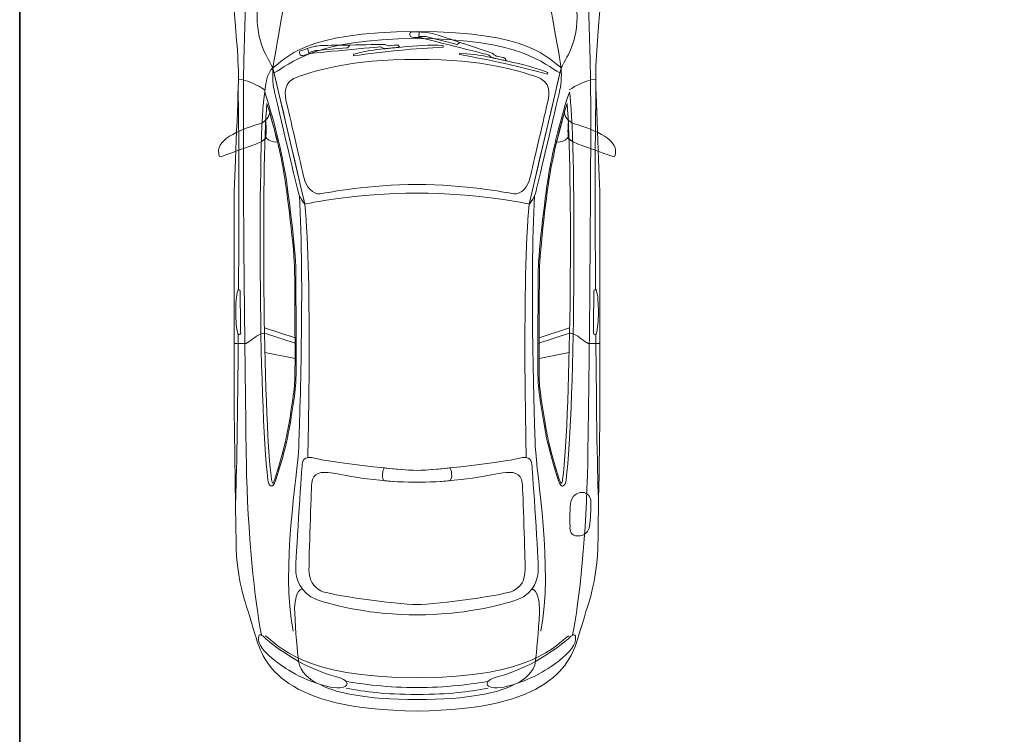
# Model space of a CAD drawing. Units: inches. Extents: x 1976 to 2558, y -977 to 2909.
# Tile 1 of 8: x 2055 to 2173, y 1884 to 1970. Entities that reach past the tile are written whole.
import ezdxf

# ---------------------------------------------------------------- set-up
doc = ezdxf.new("R2010")
doc.units = ezdxf.units.IN
doc.layers.add('A-ANNO-TTLB', color=7, linetype='Continuous', lineweight=35)
doc.layers.add('AUDI', color=7, linetype='Continuous', lineweight=18)

msp = doc.modelspace()

# ---------------------------------------------------------------- linework, layer by layer
at = {"layer": 'A-ANNO-TTLB'}
msp.add_lwpolyline([(2055.4343, 2428.9091), (2450.0007, 2428.9091), (2450.0007, 1815.3916), (2055.4343, 1815.3916)], close=True, dxfattribs=at)
at = {"layer": 'AUDI'}
for points, knots in [([(2103.0114, 1886.9558), (2086.9517, 1887.1313), (2084.6199, 1892.5316), (2083.6345, 1896.09), (2083.6345, 1896.09), (2082.9917, 1898.1907), (2082.4777, 1899.8626), (2082.2206, 1900.7202), (2082.2206, 1900.7202), (2081.9634, 1901.5775), (2081.4067, 1904.1927), (2081.3636, 1906.3792), (2081.3636, 1906.3792), (2081.3206, 1908.5657), (2081.1085, 1921.6021), (2081.1085, 1925.2), (2081.1085, 1925.2), (2081.1085, 1928.7977), (2081.1085, 1945.653), (2081.1085, 1948.0508), (2081.1085, 1948.0508), (2081.1085, 1950.4484), (2081.6208, 1960.012), (2081.6208, 1963.0558), (2081.6208, 1963.0558), (2081.6208, 1966.0998), (2081.1085, 1969.9188), (2081.1085, 1971.5013), (2081.1085, 1971.5013), (2081.1085, 1973.084), (2081.4064, 1981.4476), (2081.535, 1983.2912), (2081.535, 1983.2912), (2081.6638, 1985.1347), (2082.3541, 1986.1803), (2082.9493, 1987.4927), (2082.9493, 1987.4927), (2085.2631, 1992.5941), (2091.1759, 1995.3806), (2091.8187, 1995.8094), (2091.8187, 1995.8094), (2092.4614, 1996.2383), (2093.1437, 1996.4712), (2093.9611, 1996.4712), (2093.9611, 1996.4712), (2094.7784, 1996.4712), (2094.9894, 1996.0668), (2095.3323, 1996.1525), (2095.3323, 1996.1525), (2095.6751, 1996.2383), (2096.5292, 1996.4712), (2097.4749, 1996.4712), (2097.4749, 1996.4712), (2098.4207, 1996.4712), (2103.0114, 1996.4712), (2103.0114, 1996.4712), (2103.0114, 1996.4712), (2103.0114, 1996.4712), (2107.6023, 1996.4712), (2108.548, 1996.4712), (2108.548, 1996.4712), (2109.4939, 1996.4712), (2110.3478, 1996.2383), (2110.6907, 1996.1525), (2110.6907, 1996.1525), (2111.0335, 1996.0668), (2111.2446, 1996.4712), (2112.0619, 1996.4712), (2112.0619, 1996.4712), (2112.8792, 1996.4712), (2113.5616, 1996.2383), (2114.2043, 1995.8094), (2114.2043, 1995.8094), (2114.847, 1995.3807), (2120.7599, 1992.5941), (2123.0737, 1987.4927), (2123.0737, 1987.4927), (2123.6688, 1986.1803), (2124.3592, 1985.1347), (2124.4878, 1983.2912), (2124.4878, 1983.2912), (2124.6166, 1981.4477), (2124.9145, 1973.0839), (2124.9145, 1971.5013), (2124.9145, 1971.5013), (2124.9145, 1969.9189), (2124.4021, 1966.0998), (2124.4021, 1963.0558), (2124.4021, 1963.0558), (2124.4021, 1960.012), (2124.9145, 1950.4484), (2124.9145, 1948.0508), (2124.9145, 1948.0508), (2124.9145, 1945.653), (2124.9145, 1928.7977), (2124.9145, 1925.2), (2124.9145, 1925.2), (2124.9145, 1921.6021), (2124.7023, 1908.5656), (2124.6593, 1906.3792), (2124.6593, 1906.3792), (2124.6164, 1904.1927), (2124.0596, 1901.5775), (2123.8024, 1900.7202), (2123.8024, 1900.7202), (2123.5452, 1899.8626), (2123.0312, 1898.1907), (2122.3885, 1896.09), (2122.3885, 1896.09), (2121.4031, 1892.5316), (2119.0712, 1887.1313), (2103.0114, 1886.9558)], [0, 0, 0, 0, 0.03571429, 0.03571429, 0.03571429, 0.0357143, 0.07142857, 0.07142857, 0.07142857, 0.07142858, 0.10714286, 0.10714286, 0.10714286, 0.10714287, 0.14285714, 0.14285714, 0.14285714, 0.14285715, 0.17857143, 0.17857143, 0.17857143, 0.17857144, 0.21428571, 0.21428571, 0.21428571, 0.21428572, 0.25, 0.25, 0.25, 0.25000001, 0.28571429, 0.28571429, 0.28571429, 0.2857143, 0.32142857, 0.32142857, 0.32142857, 0.32142858, 0.35714286, 0.35714286, 0.35714286, 0.35714287, 0.39285714, 0.39285714, 0.39285714, 0.39285715, 0.42857143, 0.42857143, 0.42857143, 0.42857144, 0.46428571, 0.46428571, 0.46428571, 0.46428572, 0.5, 0.5, 0.5, 0.50000001, 0.53571429, 0.53571429, 0.53571429, 0.5357143, 0.57142857, 0.57142857, 0.57142857, 0.57142858, 0.60714286, 0.60714286, 0.60714286, 0.60714287, 0.64285714, 0.64285714, 0.64285714, 0.64285715, 0.67857143, 0.67857143, 0.67857143, 0.67857144, 0.71428571, 0.71428571, 0.71428571, 0.71428572, 0.75, 0.75, 0.75, 0.75000001, 0.78571429, 0.78571429, 0.78571429, 0.7857143, 0.82142857, 0.82142857, 0.82142857, 0.82142858, 0.85714286, 0.85714286, 0.85714286, 0.85714287, 0.89285714, 0.89285714, 0.89285714, 0.89285715, 0.92857143, 0.92857143, 0.92857143, 0.92857144, 0.96428571, 0.96428571, 0.96428571, 0.96428572, 1, 1, 1, 1]), ([(2085.7492, 1964.0106), (2085.2492, 1965.0114), (2083.6975, 1967.0084), (2083.8628, 1970.7823), (2083.8628, 1970.7823), (2084.0282, 1974.5563), (2084.6983, 1984.9688), (2085.2995, 1988.2814)], [0, 0, 0, 0, 0.5, 0.5, 0.5, 0.50000001, 1, 1, 1, 1]), ([(2120.2736, 1964.0106), (2120.7738, 1965.0114), (2122.3255, 1967.0084), (2122.1602, 1970.7823), (2122.1602, 1970.7823), (2121.9948, 1974.5563), (2121.3247, 1984.9688), (2120.7235, 1988.2814)], [0, 0, 0, 0, 0.5, 0.5, 0.5, 0.50000001, 1, 1, 1, 1]), ([(2084.3876, 1896.043), (2083.5808, 1900.0799), (2082.7216, 1908.2552), (2082.5749, 1916.7694), (2082.5749, 1916.7694), (2082.4281, 1925.2835), (2082.0616, 1958.0186), (2082.2816, 1964.9178), (2082.2816, 1964.9178), (2082.5016, 1971.8171), (2082.6247, 1980.5207), (2083.8469, 1986.4445)], [0, 0, 0, 0, 0.33333333, 0.33333333, 0.33333333, 0.33333334, 0.66666667, 0.66666667, 0.66666667, 0.66666668, 1, 1, 1, 1]), ([(2121.6353, 1896.043), (2122.4422, 1900.0799), (2123.3013, 1908.2552), (2123.448, 1916.7694), (2123.448, 1916.7694), (2123.5948, 1925.2835), (2123.9614, 1958.0186), (2123.7414, 1964.9178), (2123.7414, 1964.9178), (2123.5213, 1971.8171), (2123.3982, 1980.5207), (2122.176, 1986.4445)], [0, 0, 0, 0, 0.33333333, 0.33333333, 0.33333333, 0.33333334, 0.66666667, 0.66666667, 0.66666667, 0.66666668, 1, 1, 1, 1]), ([(2103.0114, 1948.9993), (2110.2809, 1948.9993), (2116.4404, 1947.6842), (2116.4404, 1947.6842), (2116.4404, 1947.6842), (2116.4404, 1947.6842), (2120.2736, 1964.0106), (2120.2736, 1964.0106), (2120.2736, 1964.0106), (2118.7403, 1964.997), (2116.7425, 1968.3391), (2103.0114, 1968.3391), (2103.0114, 1968.3391), (2089.2805, 1968.3391), (2087.2826, 1964.997), (2085.7493, 1964.0106), (2085.7493, 1964.0106), (2085.7493, 1964.0106), (2089.5825, 1947.6842), (2089.5825, 1947.6842), (2089.5825, 1947.6842), (2089.5825, 1947.6842), (2095.7421, 1948.9992), (2103.0114, 1948.9993)], [0, 0, 0, 0, 0.16666667, 0.16666667, 0.16666667, 0.16666668, 0.33333333, 0.33333333, 0.33333333, 0.33333334, 0.5, 0.5, 0.5, 0.50000001, 0.66666667, 0.66666667, 0.66666667, 0.66666668, 0.83333333, 0.83333333, 0.83333333, 0.83333334, 1, 1, 1, 1]), ([(2103.0114, 1948.9993), (2110.2809, 1948.9993), (2116.4404, 1947.6842), (2116.4404, 1947.6842), (2116.4404, 1947.6842), (2116.4404, 1947.6842), (2120.2736, 1964.0106), (2120.2736, 1964.0106), (2120.2736, 1964.0106), (2118.7403, 1964.997), (2116.7425, 1968.3391), (2103.0114, 1968.3391), (2103.0114, 1968.3391), (2089.2805, 1968.3391), (2087.2826, 1964.997), (2085.7493, 1964.0106), (2085.7493, 1964.0106), (2085.7493, 1964.0106), (2089.5825, 1947.6842), (2089.5825, 1947.6842), (2089.5825, 1947.6842), (2089.5825, 1947.6842), (2095.7421, 1948.9993), (2103.0114, 1948.9993)], [0, 0, 0, 0, 0.16666667, 0.16666667, 0.16666667, 0.16666668, 0.33333333, 0.33333333, 0.33333333, 0.33333334, 0.5, 0.5, 0.5, 0.50000001, 0.66666667, 0.66666667, 0.66666667, 0.66666668, 0.83333333, 0.83333333, 0.83333333, 0.83333334, 1, 1, 1, 1]), ([(2103.5089, 1968.2822), (2104.1751, 1968.2822), (2104.6611, 1968.174), (2105.2374, 1967.9938), (2105.2374, 1967.9938), (2105.6694, 1967.8678), (2112.0428, 1965.742), (2112.0428, 1965.742), (2112.0428, 1965.742), (2112.0428, 1965.742), (2112.475, 1965.3997), (2112.475, 1965.3997), (2112.475, 1965.3997), (2112.475, 1965.3997), (2113.0511, 1965.2917), (2113.3752, 1965.2199), (2113.3752, 1965.2199), (2113.6995, 1965.1299), (2113.6633, 1964.8414), (2113.6633, 1964.8414), (2113.6633, 1964.8414), (2113.6633, 1964.8414), (2111.8988, 1965.2378), (2111.8988, 1965.2378), (2111.8988, 1965.2378), (2111.8988, 1965.2378), (2111.6108, 1965.5262), (2111.6108, 1965.5262), (2111.6108, 1965.5262), (2111.6108, 1965.5262), (2103.3287, 1967.6336), (2103.3287, 1967.6336), (2103.3287, 1967.6336), (2103.3287, 1967.6336), (2103.0586, 1967.6336), (2102.6445, 1967.6336), (2102.6445, 1967.6336), (2102.2302, 1967.6515), (2102.1585, 1967.7958), (2102.1585, 1967.9577), (2102.1585, 1967.9577), (2102.1585, 1968.1379), (2102.1766, 1968.3003), (2102.4286, 1968.3003), (2102.4286, 1968.3003), (2102.6806, 1968.3182), (2103.0947, 1968.3003), (2103.5089, 1968.2822)], [0, 0, 0, 0, 0.08333333, 0.08333333, 0.08333333, 0.08333334, 0.16666667, 0.16666667, 0.16666667, 0.16666668, 0.25, 0.25, 0.25, 0.25000001, 0.33333333, 0.33333333, 0.33333333, 0.33333334, 0.41666667, 0.41666667, 0.41666667, 0.41666668, 0.5, 0.5, 0.5, 0.50000001, 0.58333333, 0.58333333, 0.58333333, 0.58333334, 0.66666667, 0.66666667, 0.66666667, 0.66666668, 0.75, 0.75, 0.75, 0.75000001, 0.83333333, 0.83333333, 0.83333333, 0.83333334, 0.91666667, 0.91666667, 0.91666667, 0.91666668, 1, 1, 1, 1]), ([(2103.2388, 1967.7597), (2103.2388, 1967.7597), (2104.0669, 1967.7416), (2104.0669, 1967.7416), (2104.0669, 1967.7416), (2104.0669, 1967.7416), (2107.8117, 1966.8048), (2107.8117, 1966.8048), (2107.8117, 1966.8048), (2107.8117, 1966.8048), (2108.118, 1967.039), (2108.118, 1967.039)], [0, 0, 0, 0, 0.33333333, 0.33333333, 0.33333333, 0.33333334, 0.66666667, 0.66666667, 0.66666667, 0.66666668, 1, 1, 1, 1]), ([(2120.1288, 1963.3943), (2118.262, 1964.3869), (2115.3769, 1967.4963), (2103.0114, 1967.4963), (2103.0114, 1967.4963), (2090.6461, 1967.4963), (2087.761, 1964.3869), (2085.8941, 1963.3942)], [0, 0, 0, 0, 0.5, 0.5, 0.5, 0.50000001, 1, 1, 1, 1]), ([(2090.1493, 1966.3904), (2090.7615, 1966.6068), (2091.2656, 1966.6607), (2091.8778, 1966.6788), (2091.8778, 1966.6788), (2092.3279, 1966.6788), (2099.0977, 1966.8048), (2099.0977, 1966.8048), (2099.0977, 1966.8048), (2099.0977, 1966.8048), (2099.6197, 1966.6246), (2099.6197, 1966.6246), (2099.6197, 1966.6246), (2099.6197, 1966.6246), (2100.2139, 1966.6968), (2100.5379, 1966.7149), (2100.5379, 1966.7149), (2100.8622, 1966.7509), (2100.916, 1966.4626), (2100.916, 1966.4626), (2100.916, 1966.4626), (2100.916, 1966.4626), (2099.1338, 1966.2825), (2099.1338, 1966.2825), (2099.1338, 1966.2825), (2099.1338, 1966.2825), (2098.6476, 1966.5167), (2098.6476, 1966.5167), (2098.6476, 1966.5167), (2098.6476, 1966.5167), (2090.1855, 1965.724), (2090.1855, 1965.724), (2090.1855, 1965.724), (2090.1855, 1965.724), (2089.9335, 1965.6341), (2089.5374, 1965.508), (2089.5374, 1965.508), (2089.1591, 1965.3819), (2089.0331, 1965.49), (2088.9791, 1965.6522), (2088.9791, 1965.6522), (2088.9249, 1965.8319), (2088.889, 1965.9767), (2089.1232, 1966.0663), (2089.1232, 1966.0663), (2089.3571, 1966.1384), (2089.7532, 1966.2644), (2090.1493, 1966.3904)], [0, 0, 0, 0, 0.08333333, 0.08333333, 0.08333333, 0.08333334, 0.16666667, 0.16666667, 0.16666667, 0.16666668, 0.25, 0.25, 0.25, 0.25000001, 0.33333333, 0.33333333, 0.33333333, 0.33333334, 0.41666667, 0.41666667, 0.41666667, 0.41666668, 0.5, 0.5, 0.5, 0.50000001, 0.58333333, 0.58333333, 0.58333333, 0.58333334, 0.66666667, 0.66666667, 0.66666667, 0.66666668, 0.75, 0.75, 0.75, 0.75000001, 0.83333333, 0.83333333, 0.83333333, 0.83333334, 0.91666667, 0.91666667, 0.91666667, 0.91666668, 1, 1, 1, 1]), ([(2090.1493, 1966.3904), (2090.7615, 1966.6068), (2091.2656, 1966.6607), (2091.8778, 1966.6788), (2091.8778, 1966.6788), (2092.3279, 1966.6788), (2099.0977, 1966.8048), (2099.0977, 1966.8048), (2099.0977, 1966.8048), (2099.0977, 1966.8048), (2099.6197, 1966.6246), (2099.6197, 1966.6246), (2099.6197, 1966.6246), (2099.6197, 1966.6246), (2100.2139, 1966.6968), (2100.5379, 1966.7149), (2100.5379, 1966.7149), (2100.8622, 1966.7509), (2100.916, 1966.4626), (2100.916, 1966.4626), (2100.916, 1966.4626), (2100.916, 1966.4626), (2099.1338, 1966.2825), (2099.1338, 1966.2825), (2099.1338, 1966.2825), (2099.1338, 1966.2825), (2098.6476, 1966.5167), (2098.6476, 1966.5167), (2098.6476, 1966.5167), (2098.6476, 1966.5167), (2090.1855, 1965.724), (2090.1855, 1965.724), (2090.1855, 1965.724), (2090.1855, 1965.724), (2089.9335, 1965.6341), (2089.5374, 1965.508), (2089.5374, 1965.508), (2089.1591, 1965.3819), (2089.0331, 1965.49), (2088.9791, 1965.6522), (2088.9791, 1965.6522), (2088.9249, 1965.8319), (2088.889, 1965.9767), (2089.1232, 1966.0663), (2089.1232, 1966.0663), (2089.3571, 1966.1384), (2089.7532, 1966.2644), (2090.1493, 1966.3904)], [0, 0, 0, 0, 0.08333333, 0.08333333, 0.08333333, 0.08333334, 0.16666667, 0.16666667, 0.16666667, 0.16666668, 0.25, 0.25, 0.25, 0.25000001, 0.33333333, 0.33333333, 0.33333333, 0.33333334, 0.41666667, 0.41666667, 0.41666667, 0.41666668, 0.5, 0.5, 0.5, 0.50000001, 0.58333333, 0.58333333, 0.58333333, 0.58333334, 0.66666667, 0.66666667, 0.66666667, 0.66666668, 0.75, 0.75, 0.75, 0.75000001, 0.83333333, 0.83333333, 0.83333333, 0.83333334, 0.91666667, 0.91666667, 0.91666667, 0.91666668, 1, 1, 1, 1]), ([(2090.0775, 1965.8141), (2090.0775, 1965.8141), (2090.8514, 1966.0664), (2090.8514, 1966.0664), (2090.8514, 1966.0664), (2090.8514, 1966.0664), (2094.7225, 1966.4085), (2094.7225, 1966.4085), (2094.7225, 1966.4085), (2094.7225, 1966.4085), (2094.9386, 1966.715), (2094.9386, 1966.715)], [0, 0, 0, 0, 0.33333333, 0.33333333, 0.33333333, 0.33333334, 0.66666667, 0.66666667, 0.66666667, 0.66666668, 1, 1, 1, 1]), ([(2106.1375, 1966.6608), (2104.589, 1966.7687), (2102.8965, 1966.6426), (2101.15, 1966.4807), (2101.15, 1966.4807), (2100.304, 1966.3904), (2099.4576, 1966.3186), (2098.6295, 1966.2282), (2098.6295, 1966.2282), (2097.4593, 1966.1203), (2096.4691, 1965.8861), (2095.3887, 1965.6341), (2095.3887, 1965.6341), (2095.3887, 1965.6341), (2095.3887, 1965.4356), (2095.3887, 1965.4356), (2095.3887, 1965.4356), (2099.0615, 1965.9584), (2102.8786, 1966.3186), (2106.1556, 1966.4626), (2106.1556, 1966.4626), (2106.1556, 1966.4626), (2106.1375, 1966.6608), (2106.1375, 1966.6608)], [0, 0, 0, 0, 0.16666667, 0.16666667, 0.16666667, 0.16666668, 0.33333333, 0.33333333, 0.33333333, 0.33333334, 0.5, 0.5, 0.5, 0.50000001, 0.66666667, 0.66666667, 0.66666667, 0.66666668, 0.83333333, 0.83333333, 0.83333333, 0.83333334, 1, 1, 1, 1]), ([(2118.6866, 1963.4363), (2117.2463, 1963.9945), (2115.6077, 1964.4089), (2113.8793, 1964.7872), (2113.8793, 1964.7872), (2113.0511, 1964.9674), (2112.223, 1965.1655), (2111.4128, 1965.3276), (2111.4128, 1965.3276), (2110.2785, 1965.5804), (2109.2521, 1965.6699), (2108.1361, 1965.7601), (2108.1361, 1965.7601), (2108.1361, 1965.7601), (2108.0819, 1965.5804), (2108.0819, 1965.5804), (2108.0819, 1965.5804), (2111.7369, 1964.9494), (2115.4639, 1964.1208), (2118.6326, 1963.2382), (2118.6326, 1963.2382), (2118.6326, 1963.2382), (2118.6866, 1963.4363), (2118.6866, 1963.4363)], [0, 0, 0, 0, 0.16666667, 0.16666667, 0.16666667, 0.16666668, 0.33333333, 0.33333333, 0.33333333, 0.33333334, 0.5, 0.5, 0.5, 0.50000001, 0.66666667, 0.66666667, 0.66666667, 0.66666668, 0.83333333, 0.83333333, 0.83333333, 0.83333334, 1, 1, 1, 1]), ([(2103.0114, 1950.0266), (2108.7817, 1950.0266), (2113.5046, 1949.0803), (2114.5979, 1948.915), (2114.5979, 1948.915), (2115.49, 1948.78), (2116.3149, 1949.745), (2116.565, 1950.9023), (2116.565, 1950.9023), (2116.815, 1952.0594), (2118.4092, 1958.8147), (2118.628, 1959.7842), (2118.628, 1959.7842), (2118.8468, 1960.7538), (2119.2219, 1962.3488), (2117.0963, 1963.0055), (2117.0963, 1963.0055), (2114.9708, 1963.6624), (2111.2135, 1965.007), (2103.0114, 1965.007), (2103.0114, 1965.007), (2094.8094, 1965.007), (2091.0522, 1963.6624), (2088.9266, 1963.0055), (2088.9266, 1963.0055), (2086.801, 1962.3489), (2087.1761, 1960.7537), (2087.395, 1959.7842), (2087.395, 1959.7842), (2087.6137, 1958.8147), (2089.2079, 1952.0593), (2089.458, 1950.9023), (2089.458, 1950.9023), (2089.7081, 1949.7451), (2090.533, 1948.78), (2091.425, 1948.915), (2091.425, 1948.915), (2092.5183, 1949.0804), (2097.2412, 1950.0266), (2103.0114, 1950.0266)], [0, 0, 0, 0, 0.1, 0.1, 0.1, 0.10000001, 0.2, 0.2, 0.2, 0.20000001, 0.3, 0.3, 0.3, 0.30000001, 0.4, 0.4, 0.4, 0.40000001, 0.5, 0.5, 0.5, 0.50000001, 0.6, 0.6, 0.6, 0.60000001, 0.7, 0.7, 0.7, 0.70000001, 0.8, 0.8, 0.8, 0.80000001, 0.9, 0.9, 0.9, 0.90000001, 1, 1, 1, 1]), ([(2085.7492, 1964.0106), (2085.7492, 1964.0106), (2089.5825, 1947.6842), (2089.5825, 1947.6842), (2089.5825, 1947.6842), (2089.5825, 1947.6842), (2088.9833, 1948.2781), (2088.7642, 1949.2095), (2088.7642, 1949.2095), (2088.5451, 1950.1409), (2086.0025, 1960.7825), (2085.8381, 1961.659), (2085.8381, 1961.659), (2085.6738, 1962.5354), (2085.7493, 1964.0106), (2085.7492, 1964.0106)], [0, 0, 0, 0, 0.25, 0.25, 0.25, 0.25000001, 0.5, 0.5, 0.5, 0.50000001, 0.75, 0.75, 0.75, 0.75000001, 1, 1, 1, 1]), ([(2085.7492, 1964.0106), (2085.7492, 1964.0106), (2089.5825, 1947.6842), (2089.5825, 1947.6842), (2089.5825, 1947.6842), (2089.5825, 1947.6842), (2088.9833, 1948.2781), (2088.7642, 1949.2095), (2088.7642, 1949.2095), (2088.5451, 1950.1409), (2086.0025, 1960.7825), (2085.8381, 1961.659), (2085.8381, 1961.659), (2085.6738, 1962.5354), (2085.7492, 1964.0106), (2085.7492, 1964.0106)], [0, 0, 0, 0, 0.25, 0.25, 0.25, 0.25000001, 0.5, 0.5, 0.5, 0.50000001, 0.75, 0.75, 0.75, 0.75000001, 1, 1, 1, 1]), ([(2120.2736, 1964.0106), (2120.2736, 1964.0106), (2116.4404, 1947.6842), (2116.4404, 1947.6842), (2116.4404, 1947.6842), (2116.4404, 1947.6842), (2117.0397, 1948.2781), (2117.2587, 1949.2095), (2117.2587, 1949.2095), (2117.4778, 1950.1409), (2120.0204, 1960.7825), (2120.1848, 1961.659), (2120.1848, 1961.659), (2120.3491, 1962.5354), (2120.2736, 1964.0106), (2120.2736, 1964.0106)], [0, 0, 0, 0, 0.25, 0.25, 0.25, 0.25000001, 0.5, 0.5, 0.5, 0.50000001, 0.75, 0.75, 0.75, 0.75000001, 1, 1, 1, 1]), ([(2085.1586, 1914.6488), (2085.2441, 1913.9773), (2085.6594, 1913.3687), (2086.1044, 1914.6488), (2086.1044, 1914.6488), (2086.5493, 1915.9289), (2087.2724, 1918.5446), (2087.4948, 1919.6576), (2087.4948, 1919.6576), (2087.7173, 1920.7704), (2088.3849, 1924.4433), (2088.4961, 1926.2799), (2088.4961, 1926.2799), (2088.6072, 1928.1164), (2088.4961, 1937.5214), (2088.4961, 1939.7473), (2088.4961, 1939.7473), (2088.4961, 1941.9735), (2087.5506, 1949.5977), (2087.2167, 1951.4341), (2087.2167, 1951.4341), (2086.8829, 1953.2706), (2086.1598, 1956.9436), (2084.7674, 1961.0809), (2084.7674, 1961.0809), (2083.9351, 1956.4985), (2084.046, 1923.386), (2085.1586, 1914.6488)], [0, 0, 0, 0, 0.14285714, 0.14285714, 0.14285714, 0.14285715, 0.28571429, 0.28571429, 0.28571429, 0.2857143, 0.42857143, 0.42857143, 0.42857143, 0.42857144, 0.57142857, 0.57142857, 0.57142857, 0.57142858, 0.71428571, 0.71428571, 0.71428571, 0.71428572, 0.85714286, 0.85714286, 0.85714286, 0.85714287, 1, 1, 1, 1]), ([(2120.8644, 1914.6488), (2120.7789, 1913.9773), (2120.3635, 1913.3687), (2119.9186, 1914.6488), (2119.9186, 1914.6488), (2119.4736, 1915.9289), (2118.7506, 1918.5446), (2118.5281, 1919.6576), (2118.5281, 1919.6576), (2118.3057, 1920.7704), (2117.638, 1924.4433), (2117.5269, 1926.2799), (2117.5269, 1926.2799), (2117.4157, 1928.1164), (2117.5269, 1937.5214), (2117.5269, 1939.7473), (2117.5269, 1939.7473), (2117.5269, 1941.9735), (2118.4724, 1949.5977), (2118.8063, 1951.4341), (2118.8063, 1951.4341), (2119.1401, 1953.2706), (2119.8632, 1956.9436), (2121.2556, 1961.0809), (2121.2556, 1961.0809), (2122.0879, 1956.4985), (2121.977, 1923.386), (2120.8644, 1914.6488)], [0, 0, 0, 0, 0.14285714, 0.14285714, 0.14285714, 0.14285715, 0.28571429, 0.28571429, 0.28571429, 0.2857143, 0.42857143, 0.42857143, 0.42857143, 0.42857144, 0.57142857, 0.57142857, 0.57142857, 0.57142858, 0.71428571, 0.71428571, 0.71428571, 0.71428572, 0.85714286, 0.85714286, 0.85714286, 0.85714287, 1, 1, 1, 1]), ([(2085.5815, 1914.6846), (2085.5815, 1914.6846), (2085.5815, 1914.6846), (2085.5815, 1914.6846), (2085.5815, 1914.6846), (2085.6128, 1914.4387), (2085.6797, 1914.296), (2085.7283, 1914.2272), (2085.7283, 1914.2272), (2085.7791, 1914.2878), (2085.8668, 1914.4215), (2085.9781, 1914.742), (2085.9781, 1914.742), (2086.4118, 1915.9895), (2087.1342, 1918.5913), (2087.3583, 1919.7131), (2087.3583, 1919.7131), (2087.627, 1921.057), (2088.2509, 1924.5803), (2088.3547, 1926.2969), (2088.3547, 1926.2969), (2088.436, 1927.64), (2088.3969, 1933.128), (2088.3713, 1936.7597), (2088.3713, 1936.7597), (2088.3713, 1936.7597), (2088.3542, 1939.7474), (2088.3542, 1939.7474), (2088.3542, 1939.7474), (2088.3542, 1941.9672), (2087.3984, 1949.628), (2087.0795, 1951.3834), (2087.0795, 1951.3834), (2086.5458, 1954.3188), (2085.8538, 1957.1139), (2085.0352, 1959.7351), (2085.0352, 1959.7351), (2084.3813, 1952.1416), (2084.5505, 1922.7803), (2085.5815, 1914.6846)], [0, 0, 0, 0, 0.1, 0.1, 0.1, 0.10000001, 0.2, 0.2, 0.2, 0.20000001, 0.3, 0.3, 0.3, 0.30000001, 0.4, 0.4, 0.4, 0.40000001, 0.5, 0.5, 0.5, 0.50000001, 0.6, 0.6, 0.6, 0.60000001, 0.7, 0.7, 0.7, 0.70000001, 0.8, 0.8, 0.8, 0.80000001, 0.9, 0.9, 0.9, 0.90000001, 1, 1, 1, 1]), ([(2120.4414, 1914.6846), (2120.4414, 1914.6846), (2120.4414, 1914.6846), (2120.4414, 1914.6846), (2120.4414, 1914.6846), (2120.4102, 1914.4387), (2120.3433, 1914.296), (2120.2947, 1914.2272), (2120.2947, 1914.2272), (2120.2439, 1914.2878), (2120.1562, 1914.4215), (2120.0448, 1914.742), (2120.0448, 1914.742), (2119.6112, 1915.9895), (2118.8888, 1918.5913), (2118.6646, 1919.7131), (2118.6646, 1919.7131), (2118.396, 1921.057), (2117.7721, 1924.5803), (2117.6683, 1926.2969), (2117.6683, 1926.2969), (2117.5869, 1927.64), (2117.626, 1933.128), (2117.6516, 1936.7597), (2117.6516, 1936.7597), (2117.6516, 1936.7597), (2117.6688, 1939.7474), (2117.6688, 1939.7474), (2117.6688, 1939.7474), (2117.6688, 1941.9672), (2118.6246, 1949.628), (2118.9435, 1951.3834), (2118.9435, 1951.3834), (2119.477, 1954.3188), (2120.1692, 1957.1139), (2120.9877, 1959.7351), (2120.9877, 1959.7351), (2121.6417, 1952.1416), (2121.4724, 1922.7803), (2120.4414, 1914.6846)], [0, 0, 0, 0, 0.1, 0.1, 0.1, 0.10000001, 0.2, 0.2, 0.2, 0.20000001, 0.3, 0.3, 0.3, 0.30000001, 0.4, 0.4, 0.4, 0.40000001, 0.5, 0.5, 0.5, 0.50000001, 0.6, 0.6, 0.6, 0.60000001, 0.7, 0.7, 0.7, 0.70000001, 0.8, 0.8, 0.8, 0.80000001, 0.9, 0.9, 0.9, 0.90000001, 1, 1, 1, 1]), ([(2084.8602, 1957.7124), (2084.9485, 1957.2548), (2084.9566, 1956.2582), (2084.9031, 1955.5721), (2084.9031, 1955.5721), (2084.9229, 1955.594), (2084.9449, 1955.6162), (2084.9583, 1955.6357), (2084.9583, 1955.6357), (2085.0814, 1955.3744), (2085.7149, 1955.0296), (2086.2973, 1955.1251), (2086.2973, 1955.1251), (2086.2208, 1955.4446), (2085.37, 1958.6289), (2085.37, 1958.6289), (2085.37, 1958.6289), (2085.3354, 1958.3654), (2085.1696, 1958.0077), (2084.8602, 1957.7124)], [0, 0, 0, 0, 0.2, 0.2, 0.2, 0.20000001, 0.4, 0.4, 0.4, 0.40000001, 0.6, 0.6, 0.6, 0.60000001, 0.8, 0.8, 0.8, 0.80000001, 1, 1, 1, 1]), ([(2121.1628, 1957.7124), (2121.0744, 1957.2548), (2121.0663, 1956.2582), (2121.1199, 1955.5721), (2121.1199, 1955.5721), (2121.1001, 1955.594), (2121.0781, 1955.6162), (2121.0646, 1955.6357), (2121.0646, 1955.6357), (2120.9416, 1955.3744), (2120.3081, 1955.0296), (2119.7257, 1955.1251), (2119.7257, 1955.1251), (2119.8021, 1955.4446), (2120.6529, 1958.6289), (2120.6529, 1958.6289), (2120.6529, 1958.6289), (2120.6876, 1958.3654), (2120.8534, 1958.0077), (2121.1628, 1957.7124)], [0, 0, 0, 0, 0.2, 0.2, 0.2, 0.20000001, 0.4, 0.4, 0.4, 0.40000001, 0.6, 0.6, 0.6, 0.60000001, 0.8, 0.8, 0.8, 0.80000001, 1, 1, 1, 1]), ([(2084.8602, 1957.7124), (2084.6525, 1957.5142), (2084.382, 1957.3434), (2084.0362, 1957.2506), (2084.0362, 1957.2506), (2083.1754, 1957.0196), (2079.3023, 1955.8051), (2079.2562, 1954.1441), (2079.2562, 1954.1441), (2079.2562, 1953.4367), (2079.2714, 1953.1907), (2079.8247, 1953.4366), (2079.8247, 1953.4366), (2080.3781, 1953.6828), (2083.1603, 1954.6821), (2083.6213, 1954.8206), (2083.6213, 1954.8206), (2084.0458, 1954.9483), (2084.6733, 1955.3214), (2084.9031, 1955.5721), (2084.9031, 1955.5721), (2084.9566, 1956.2582), (2084.9485, 1957.2548), (2084.8602, 1957.7124)], [0, 0, 0, 0, 0.16666667, 0.16666667, 0.16666667, 0.16666668, 0.33333333, 0.33333333, 0.33333333, 0.33333334, 0.5, 0.5, 0.5, 0.50000001, 0.66666667, 0.66666667, 0.66666667, 0.66666668, 0.83333333, 0.83333333, 0.83333333, 0.83333334, 1, 1, 1, 1]), ([(2121.1628, 1957.7124), (2121.3704, 1957.5142), (2121.6409, 1957.3434), (2121.9868, 1957.2506), (2121.9868, 1957.2506), (2122.8475, 1957.0196), (2126.7206, 1955.8051), (2126.7668, 1954.1441), (2126.7668, 1954.1441), (2126.7668, 1953.4367), (2126.7516, 1953.1907), (2126.1983, 1953.4366), (2126.1983, 1953.4366), (2125.6449, 1953.6828), (2122.8627, 1954.6821), (2122.4017, 1954.8206), (2122.4017, 1954.8206), (2121.9772, 1954.9483), (2121.3496, 1955.3214), (2121.1199, 1955.5721), (2121.1199, 1955.5721), (2121.0663, 1956.2582), (2121.0744, 1957.2548), (2121.1628, 1957.7124)], [0, 0, 0, 0, 0.16666667, 0.16666667, 0.16666667, 0.16666668, 0.33333333, 0.33333333, 0.33333333, 0.33333334, 0.5, 0.5, 0.5, 0.50000001, 0.66666667, 0.66666667, 0.66666667, 0.66666668, 0.83333333, 0.83333333, 0.83333333, 0.83333334, 1, 1, 1, 1]), ([(2088.9388, 1948.6826), (2089.5144, 1938.2955), (2088.9728, 1921.9609), (2088.8477, 1918.6458), (2088.8477, 1918.6458), (2088.7227, 1915.3308), (2086.6936, 1904.0712), (2088.1806, 1896.5372)], [0, 0, 0, 0, 0.5, 0.5, 0.5, 0.50000001, 1, 1, 1, 1]), ([(2117.0841, 1948.6826), (2116.5086, 1938.2955), (2117.0502, 1921.9609), (2117.1752, 1918.6458), (2117.1752, 1918.6458), (2117.3003, 1915.3308), (2119.3293, 1904.0712), (2117.8424, 1896.5372)], [0, 0, 0, 0, 0.5, 0.5, 0.5, 0.50000001, 1, 1, 1, 1]), ([(2081.8933, 1932.2234), (2081.8933, 1932.0271), (2081.6249, 1931.9534), (2081.5654, 1932.1498), (2081.5654, 1932.1498), (2081.3861, 1932.7144), (2081.2972, 1933.7203), (2081.2972, 1934.7265), (2081.2972, 1934.7265), (2081.2972, 1935.7327), (2081.3566, 1936.7143), (2081.5353, 1937.3033), (2081.5353, 1937.3033), (2081.5949, 1937.4751), (2081.8333, 1937.4259), (2081.8333, 1937.2295), (2081.8333, 1937.2295), (2081.8333, 1937.2295), (2081.8933, 1932.2234), (2081.8933, 1932.2234)], [0, 0, 0, 0, 0.2, 0.2, 0.2, 0.20000001, 0.4, 0.4, 0.4, 0.40000001, 0.6, 0.6, 0.6, 0.60000001, 0.8, 0.8, 0.8, 0.80000001, 1, 1, 1, 1]), ([(2124.1296, 1932.2234), (2124.1296, 1932.0271), (2124.398, 1931.9534), (2124.4576, 1932.1498), (2124.4576, 1932.1498), (2124.6368, 1932.7144), (2124.7257, 1933.7203), (2124.7257, 1934.7265), (2124.7257, 1934.7265), (2124.7257, 1935.7327), (2124.6664, 1936.7143), (2124.4876, 1937.3033), (2124.4876, 1937.3033), (2124.428, 1937.4751), (2124.1897, 1937.4259), (2124.1897, 1937.2295), (2124.1897, 1937.2295), (2124.1897, 1937.2295), (2124.1296, 1932.2234), (2124.1296, 1932.2234)], [0, 0, 0, 0, 0.2, 0.2, 0.2, 0.20000001, 0.4, 0.4, 0.4, 0.40000001, 0.6, 0.6, 0.6, 0.60000001, 0.8, 0.8, 0.8, 0.80000001, 1, 1, 1, 1]), ([(2081.1085, 1930.9631), (2081.1085, 1930.9631), (2082.0736, 1930.963), (2082.3905, 1930.963), (2082.3905, 1930.963), (2082.7075, 1930.963), (2083.5476, 1931.7317), (2083.9351, 1931.9563), (2083.9351, 1931.9563), (2084.3226, 1932.181), (2084.7483, 1932.2343), (2084.7483, 1932.2343)], [0, 0, 0, 0, 0.33333333, 0.33333333, 0.33333333, 0.33333334, 0.66666667, 0.66666667, 0.66666667, 0.66666668, 1, 1, 1, 1]), ([(2124.9145, 1930.9631), (2124.9145, 1930.9631), (2123.9494, 1930.963), (2123.6324, 1930.963), (2123.6324, 1930.963), (2123.3154, 1930.963), (2122.4754, 1931.7317), (2122.0879, 1931.9563), (2122.0879, 1931.9563), (2121.7003, 1932.181), (2121.2747, 1932.2343), (2121.2747, 1932.2343)], [0, 0, 0, 0, 0.33333333, 0.33333333, 0.33333333, 0.33333334, 0.66666667, 0.66666667, 0.66666667, 0.66666668, 1, 1, 1, 1]), ([(2103.0114, 1898.4759), (2108.4108, 1898.4759), (2112.9495, 1899.5599), (2115.0333, 1900.3106), (2115.0333, 1900.3106), (2117.1171, 1901.0612), (2117.534, 1902.9794), (2117.534, 1903.9384), (2117.534, 1903.9384), (2117.534, 1904.8975), (2116.867, 1915.4474), (2116.7837, 1916.1981), (2116.7837, 1916.1981), (2116.7005, 1916.9487), (2116.742, 1917.6159), (2115.1166, 1917.1988), (2115.1166, 1917.1988), (2113.4912, 1916.7817), (2105.0308, 1915.7811), (2103.0114, 1915.7811), (2103.0114, 1915.7811), (2100.9922, 1915.7811), (2092.5318, 1916.7817), (2090.9064, 1917.1988), (2090.9064, 1917.1988), (2089.2809, 1917.6159), (2089.3224, 1916.9487), (2089.2392, 1916.1981), (2089.2392, 1916.1981), (2089.1559, 1915.4474), (2088.489, 1904.8974), (2088.489, 1903.9384), (2088.489, 1903.9384), (2088.489, 1902.9794), (2088.9059, 1901.0612), (2090.9896, 1900.3106), (2090.9896, 1900.3106), (2093.0734, 1899.5599), (2097.6121, 1898.4759), (2103.0114, 1898.4759)], [0, 0, 0, 0, 0.1, 0.1, 0.1, 0.10000001, 0.2, 0.2, 0.2, 0.20000001, 0.3, 0.3, 0.3, 0.30000001, 0.4, 0.4, 0.4, 0.40000001, 0.5, 0.5, 0.5, 0.50000001, 0.6, 0.6, 0.6, 0.60000001, 0.7, 0.7, 0.7, 0.70000001, 0.8, 0.8, 0.8, 0.80000001, 0.9, 0.9, 0.9, 0.90000001, 1, 1, 1, 1]), ([(2103.0114, 1898.4759), (2108.4108, 1898.4759), (2112.9495, 1899.5599), (2115.0333, 1900.3106), (2115.0333, 1900.3106), (2117.1171, 1901.0612), (2117.534, 1902.9794), (2117.534, 1903.9384), (2117.534, 1903.9384), (2117.534, 1904.8975), (2116.867, 1915.4474), (2116.7837, 1916.1981), (2116.7837, 1916.1981), (2116.7005, 1916.9487), (2116.742, 1917.6159), (2115.1166, 1917.1988), (2115.1166, 1917.1988), (2113.4912, 1916.7817), (2105.0308, 1915.7811), (2103.0114, 1915.7811), (2103.0114, 1915.7811), (2100.9922, 1915.7811), (2092.5318, 1916.7817), (2090.9064, 1917.1988), (2090.9064, 1917.1988), (2089.2809, 1917.6159), (2089.3224, 1916.9487), (2089.2392, 1916.1981), (2089.2392, 1916.1981), (2089.1559, 1915.4474), (2088.489, 1904.8974), (2088.489, 1903.9384), (2088.489, 1903.9384), (2088.489, 1902.9794), (2088.9059, 1901.0612), (2090.9896, 1900.3106), (2090.9896, 1900.3106), (2093.0734, 1899.5599), (2097.6121, 1898.4759), (2103.0114, 1898.4759)], [0, 0, 0, 0, 0.1, 0.1, 0.1, 0.10000001, 0.2, 0.2, 0.2, 0.20000001, 0.3, 0.3, 0.3, 0.30000001, 0.4, 0.4, 0.4, 0.40000001, 0.5, 0.5, 0.5, 0.50000001, 0.6, 0.6, 0.6, 0.60000001, 0.7, 0.7, 0.7, 0.70000001, 0.8, 0.8, 0.8, 0.80000001, 0.9, 0.9, 0.9, 0.90000001, 1, 1, 1, 1]), ([(2103.0114, 1914.3634), (2103.0114, 1914.3634), (2106.0696, 1914.4171), (2106.8672, 1914.5347), (2106.8672, 1914.5347), (2107.3661, 1914.6084), (2107.1314, 1916.1003), (2106.8982, 1916.0777), (2106.8982, 1916.0777), (2105.4327, 1915.9354), (2104.2005, 1915.7811), (2103.0114, 1915.7811), (2103.0114, 1915.7811), (2101.8224, 1915.7811), (2100.5902, 1915.9354), (2099.1248, 1916.0777), (2099.1248, 1916.0777), (2098.8915, 1916.1003), (2098.6569, 1914.6083), (2099.1558, 1914.5347), (2099.1558, 1914.5347), (2099.9533, 1914.4171), (2103.0114, 1914.3634), (2103.0114, 1914.3634)], [0, 0, 0, 0, 0.16666667, 0.16666667, 0.16666667, 0.16666668, 0.33333333, 0.33333333, 0.33333333, 0.33333334, 0.5, 0.5, 0.5, 0.50000001, 0.66666667, 0.66666667, 0.66666667, 0.66666668, 0.83333333, 0.83333333, 0.83333333, 0.83333334, 1, 1, 1, 1]), ([(2103.0114, 1899.7242), (2105.5726, 1899.7242), (2113.6162, 1900.8527), (2114.5332, 1901.3531), (2114.5332, 1901.3531), (2115.4502, 1901.8535), (2115.9503, 1902.5623), (2115.9503, 1903.9384), (2115.9503, 1903.9384), (2115.9503, 1905.3145), (2115.7, 1913.0289), (2115.6167, 1914.2799), (2115.6167, 1914.2799), (2115.5334, 1915.5309), (2114.4082, 1915.656), (2113.2829, 1915.4892), (2113.2829, 1915.4892), (2112.1576, 1915.3224), (2108.1983, 1914.3634), (2103.0114, 1914.3634), (2103.0114, 1914.3634), (2097.8246, 1914.3634), (2093.8653, 1915.3224), (2092.7401, 1915.4892), (2092.7401, 1915.4892), (2091.6148, 1915.656), (2090.4895, 1915.5309), (2090.4062, 1914.2799), (2090.4062, 1914.2799), (2090.3229, 1913.029), (2090.0726, 1905.3145), (2090.0726, 1903.9384), (2090.0726, 1903.9384), (2090.0726, 1902.5623), (2090.5728, 1901.8535), (2091.4897, 1901.3531), (2091.4897, 1901.3531), (2092.4067, 1900.8528), (2100.4503, 1899.7242), (2103.0114, 1899.7242)], [0, 0, 0, 0, 0.1, 0.1, 0.1, 0.10000001, 0.2, 0.2, 0.2, 0.20000001, 0.3, 0.3, 0.3, 0.30000001, 0.4, 0.4, 0.4, 0.40000001, 0.5, 0.5, 0.5, 0.50000001, 0.6, 0.6, 0.6, 0.60000001, 0.7, 0.7, 0.7, 0.70000001, 0.8, 0.8, 0.8, 0.80000001, 0.9, 0.9, 0.9, 0.90000001, 1, 1, 1, 1]), ([(2121.3313, 1909.0484), (2121.2734, 1908.5035), (2121.4685, 1907.9385), (2122.2592, 1907.9234), (2122.2592, 1907.9234), (2123.05, 1907.9082), (2123.5931, 1908.3294), (2123.7091, 1909.3738), (2123.7091, 1909.3738), (2123.8251, 1910.4182), (2123.8251, 1911.4625), (2123.8251, 1912.0428), (2123.8251, 1912.0428), (2123.8251, 1912.6231), (2123.419, 1913.1452), (2122.7812, 1913.1452), (2122.7812, 1913.1452), (2122.1433, 1913.1452), (2121.5055, 1912.7392), (2121.3894, 1911.8108), (2121.3894, 1911.8108), (2121.2734, 1910.8824), (2121.3313, 1909.0484), (2121.3313, 1909.0484)], [0, 0, 0, 0, 0.16666667, 0.16666667, 0.16666667, 0.16666668, 0.33333333, 0.33333333, 0.33333333, 0.33333334, 0.5, 0.5, 0.5, 0.50000001, 0.66666667, 0.66666667, 0.66666667, 0.66666668, 0.83333333, 0.83333333, 0.83333333, 0.83333334, 1, 1, 1, 1]), ([(2088.8231, 1892.914), (2088.7, 1893.9427), (2088.4565, 1896.5748), (2088.364, 1898.7052), (2088.364, 1898.7052), (2088.3014, 1900.1438), (2088.6101, 1901.4262), (2089.2372, 1901.5981)], [0, 0, 0, 0, 0.5, 0.5, 0.5, 0.50000001, 1, 1, 1, 1]), ([(2117.1999, 1892.914), (2117.3229, 1893.9427), (2117.5664, 1896.5748), (2117.659, 1898.7052), (2117.659, 1898.7052), (2117.7215, 1900.1438), (2117.4128, 1901.4262), (2116.7857, 1901.5981)], [0, 0, 0, 0, 0.5, 0.5, 0.5, 0.50000001, 1, 1, 1, 1]), ([(2093.3706, 1891.0589), (2088.9181, 1892.2105), (2085.312, 1895.2117), (2084.7559, 1895.7516), (2084.7559, 1895.7516), (2084.2665, 1896.2269), (2083.9659, 1896.279), (2084.0423, 1895.4419), (2084.0423, 1895.4419), (2084.1178, 1894.616), (2085.1591, 1893.6856), (2085.7982, 1893.1555), (2085.7982, 1893.1555), (2086.6145, 1892.4783), (2088.8555, 1890.7878), (2092.1665, 1889.9447), (2092.1665, 1889.9447), (2093.4307, 1889.5833), (2094.3337, 1889.7038), (2094.5745, 1890.0651), (2094.5745, 1890.0651), (2094.8153, 1890.4265), (2094.2548, 1890.8291), (2093.3706, 1891.0589)], [0, 0, 0, 0, 0.16666667, 0.16666667, 0.16666667, 0.16666668, 0.33333333, 0.33333333, 0.33333333, 0.33333334, 0.5, 0.5, 0.5, 0.50000001, 0.66666667, 0.66666667, 0.66666667, 0.66666668, 0.83333333, 0.83333333, 0.83333333, 0.83333334, 1, 1, 1, 1]), ([(2121.1904, 1895.9832), (2119.597, 1894.8897), (2116.8712, 1890.9491), (2103.0114, 1890.9491), (2103.0114, 1890.9491), (2089.1518, 1890.9491), (2086.426, 1894.8897), (2084.8326, 1895.9832)], [0, 0, 0, 0, 0.5, 0.5, 0.5, 0.50000001, 1, 1, 1, 1]), ([(2112.6523, 1891.0589), (2117.1049, 1892.2105), (2120.7111, 1895.2117), (2121.2671, 1895.7516), (2121.2671, 1895.7516), (2121.7565, 1896.2269), (2122.0571, 1896.279), (2121.9806, 1895.4419), (2121.9806, 1895.4419), (2121.9052, 1894.616), (2120.8639, 1893.6856), (2120.2249, 1893.1555), (2120.2249, 1893.1555), (2119.4084, 1892.4783), (2117.1674, 1890.7878), (2113.8565, 1889.9447), (2113.8565, 1889.9447), (2112.5923, 1889.5833), (2111.6892, 1889.7038), (2111.4484, 1890.0651), (2111.4484, 1890.0651), (2111.2076, 1890.4265), (2111.7681, 1890.8291), (2112.6523, 1891.0589)], [0, 0, 0, 0, 0.16666667, 0.16666667, 0.16666667, 0.16666668, 0.33333333, 0.33333333, 0.33333333, 0.33333334, 0.5, 0.5, 0.5, 0.50000001, 0.66666667, 0.66666667, 0.66666667, 0.66666668, 0.83333333, 0.83333333, 0.83333333, 0.83333334, 1, 1, 1, 1]), ([(2114.7053, 1890.1861), (2113.1579, 1889.198), (2109.1192, 1888.3223), (2103.0114, 1888.3223), (2103.0114, 1888.3223), (2096.9037, 1888.3223), (2092.8651, 1889.198), (2091.3176, 1890.1861)], [0, 0, 0, 0, 0.5, 0.5, 0.5, 0.50000001, 1, 1, 1, 1]), ([(2111.5153, 1890.5048), (2109.907, 1890.1986), (2106.2435, 1889.7607), (2103.0114, 1889.7607), (2103.0114, 1889.7607), (2099.7794, 1889.7607), (2096.1159, 1890.1986), (2094.5076, 1890.5048)], [0, 0, 0, 0, 0.5, 0.5, 0.5, 0.50000001, 1, 1, 1, 1]), ([(2111.5153, 1889.6982), (2109.0318, 1889.2605), (2107.0562, 1888.9477), (2103.0114, 1888.9477), (2103.0114, 1888.9477), (2098.9667, 1888.9477), (2096.9911, 1889.2605), (2094.5076, 1889.6982)], [0, 0, 0, 0, 0.5, 0.5, 0.5, 0.50000001, 1, 1, 1, 1])]:
    msp.add_open_spline(points, degree=3, knots=knots, dxfattribs=at)
for points in [[(2091.6954, 1993.6315), (2090.2812, 1989.1303), (2085.9918, 1966.0704), (2085.7417, 1963.8187)], [(2114.3276, 1993.6315), (2115.7417, 1989.1303), (2120.0311, 1966.0704), (2120.2812, 1963.8187)], [(2103.2388, 1967.6336), (2103.2388, 1967.6336), (2103.2566, 1968.3003), (2103.2566, 1968.3003)], [(2090.1134, 1965.6881), (2090.1134, 1965.6881), (2089.897, 1966.3186), (2089.897, 1966.3186)], [(2084.738, 1960.8162), (2084.8213, 1961.567), (2084.9986, 1963.4343), (2085.7493, 1964.0106)], [(2084.7978, 1961.3406), (2084.7978, 1961.3406), (2082.9989, 1962.6089), (2081.6178, 1962.6089)], [(2121.2251, 1961.3406), (2121.2251, 1961.3406), (2123.0242, 1962.6089), (2124.4051, 1962.6089)], [(2081.6401, 1937.4023), (2081.695, 1947.3511), (2081.6887, 1957.2442), (2081.5879, 1961.2274)], [(2124.3829, 1937.4023), (2124.3279, 1947.3511), (2124.3343, 1957.2442), (2124.4351, 1961.2274)], [(2089.9342, 1917.3201), (2089.9342, 1917.3201), (2090.4678, 1938.597), (2089.5825, 1947.6842)], [(2116.0888, 1917.3201), (2116.0888, 1917.3201), (2115.5552, 1938.597), (2116.4404, 1947.6842)], [(2084.7375, 1932.8406), (2084.7375, 1932.8406), (2088.4008, 1931.6378), (2088.4008, 1931.6378)], [(2121.2854, 1932.8406), (2121.2854, 1932.8406), (2117.6222, 1931.6378), (2117.6222, 1931.6378)], [(2081.2702, 1911.963), (2081.4125, 1914.5033), (2081.5333, 1922.8492), (2081.6049, 1932.08)], [(2084.7483, 1932.2343), (2084.7483, 1932.2343), (2088.5444, 1930.9631), (2088.5444, 1930.9631)], [(2121.2747, 1932.2343), (2121.2747, 1932.2343), (2117.4785, 1930.9631), (2117.4785, 1930.9631)], [(2124.7528, 1911.963), (2124.6105, 1914.5033), (2124.4895, 1922.8492), (2124.418, 1932.08)], [(2084.7966, 1929.894), (2084.7966, 1929.894), (2088.4023, 1929.1734), (2088.4023, 1929.1734)], [(2121.2263, 1929.894), (2121.2263, 1929.894), (2117.6207, 1929.1734), (2117.6207, 1929.1734)], [(2088.8231, 1892.914), (2088.9635, 1891.5965), (2090.2556, 1890.6569), (2091.0961, 1890.2572)], [(2117.1999, 1892.914), (2117.0595, 1891.5965), (2115.7674, 1890.6569), (2114.9269, 1890.2572)]]:
    msp.add_open_spline(points, degree=3, dxfattribs=at)

doc.saveas('drawing.dxf')
